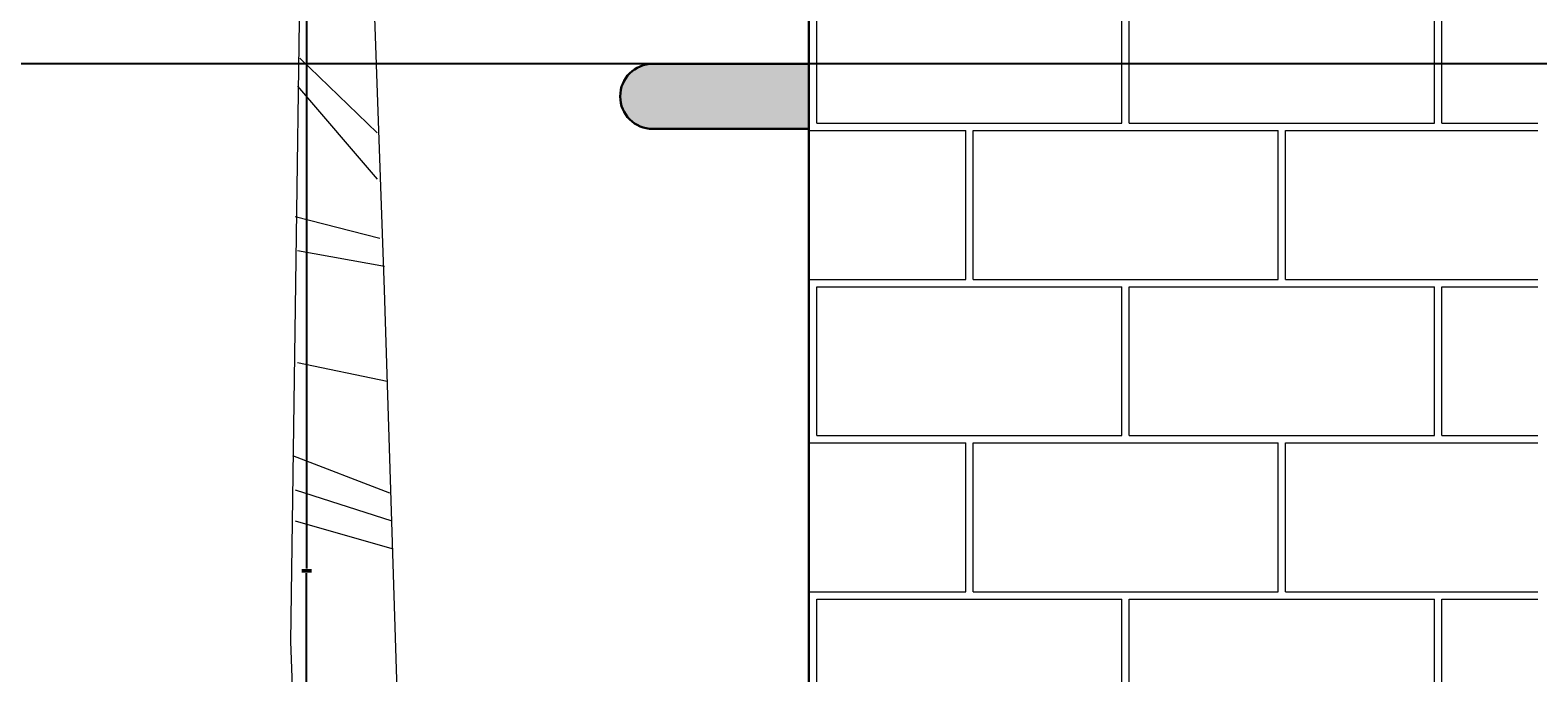
# Model space of a CAD drawing. Units: inches. Extents: x -301 to 715, y -607 to 364.
# Tile 129 of 141: x 194 to 310, y -440 to -391. Entities that reach past the tile are written whole.
import ezdxf

# ---------------------------------------------------------------- set-up
doc = ezdxf.new("R2010")
doc.units = ezdxf.units.IN
doc.header["$MEASUREMENT"] = 0
for name, color, linetype, lineweight in [('A-ANNO-DIMS', 2, 'Continuous', 18), ('A-ELEV', 220, 'Continuous', 30), ('A-ELEV-PATT', 4, 'Continuous', 13), ('L-PLNT', 94, 'Continuous', 13)]:
    doc.layers.add(name, color=color, linetype=linetype, lineweight=lineweight)
doc.styles.get("Standard").update_dxf_attribs({"font": 'arial.ttf'})
doc.dimstyles.get("Standard").update_dxf_attribs({"dimtxt": 0.18, "dimasz": 0.18, "dimexe": 0.18, "dimexo": 0.0625, "dimgap": 0.09, "dimtad": 0, "dimtih": 1, "dimtoh": 1, "dimdec": 1, "dimzin": 0, "dimdsep": 46, "dimlunit": 4, "dimtxsty": 'Standard', "dimcen": 0.09, "dimclrd": 3, "dimclre": 4, "dimclrt": 6, "dimadec": 0, "dimazin": 0, "dimtfac": 1, "dimtdec": 1, "dimtofl": 0, "dimtmove": 0, "dimatfit": 3, "dimfxl": 1, "dimtfill": 2, "dimtfillclr": 51, "dimtolj": 1, "dimtzin": 0, "dimarcsym": 0})

# ---------------------------------------------------------------- blocks, each defined once
blk = doc.blocks.new('*U34')
for p, q in [((-4.267, 114.428), (1.682, 108.708)), ((-4.453, 112.283), (1.682, 105.133)), ((-4.639, 102.273), (1.868, 100.604)), ((-4.453, 99.651), (2.24, 98.459)), ((-4.453, 91.071), (2.426, 89.641)), ((-4.825, 83.921), (2.612, 81.061)), ((-4.639, 81.299), (2.797, 78.916)), ((-4.639, 78.916), (2.797, 76.771))]:
    blk.add_line(p, q)
for points in [[(-2.363, 170.553), (-3.88, 148.505), (-4.988, 69.634), (-3.325, 24.869), (0, 0)], [(-0.116, 162.848), (0.554, 143.532), (2.217, 96.635), (3.88, 44.054), (7.76, 12.079), (11.64, 0)]]:
    blk.add_lwpolyline(points)
blk = doc.blocks.new('*D176')
at = {"layer": 'A-ANNO-DIMS', "color": 4, "lineweight": -2, "transparency": 16777216}
for p, q in [((148.28, -324.48), (215.61, -324.48)), ((-15.22, -540.48), (215.61, -540.48))]:
    blk.add_line(p, q, dxfattribs=at)
at = {"layer": 'A-ANNO-DIMS', "color": 3, "lineweight": -2, "transparency": 16777216}
for p, q in [((215.43, -324.66), (215.43, -432.3)), ((215.43, -540.3), (215.43, -432.66))]:
    blk.add_line(p, q, dxfattribs=at)
at = {"layer": 'A-ANNO-DIMS', "color": 3, "transparency": 16777216}
for points in [[(215.4, -324.66), (215.46, -324.66), (215.43, -324.48)], [(215.4, -540.3), (215.46, -540.3), (215.43, -540.48)]]:
    blk.add_solid(points, dxfattribs=at)
at = {"layer": 'Defpoints', "color": 0, "transparency": 16777216}
for p in [(148.22, -324.48), (-15.28, -540.48), (215.43, -540.48)]:
    blk.add_point(p, dxfattribs=at)
at = {"layer": 'A-ANNO-DIMS', "color": 6, "transparency": 16777216, "insert": (215.43, -432.48), "char_height": 0.18, "attachment_point": 5, "bg_fill": 1, "box_fill_scale": 1.25, "bg_fill_color": 51, "bg_fill_transparency": 0}
blk.add_mtext('\\A1;18\'-0"', dxfattribs=at)
blk = doc.blocks.new('*D200')
at = {"layer": 'A-ANNO-DIMS', "color": 4, "lineweight": -2, "transparency": 16777216}
for p, q in [((412.96, -393.55), (121.93, -393.55)), ((412.96, -489.55), (121.93, -489.55))]:
    blk.add_line(p, q, dxfattribs=at)
at = {"layer": 'A-ANNO-DIMS', "color": 3, "lineweight": -2, "transparency": 16777216}
for p, q in [((122.11, -393.73), (122.11, -441.37)), ((122.11, -489.37), (122.11, -441.73))]:
    blk.add_line(p, q, dxfattribs=at)
at = {"layer": 'A-ANNO-DIMS', "color": 3, "transparency": 16777216}
for points in [[(122.08, -393.73), (122.14, -393.73), (122.11, -393.55)], [(122.08, -489.37), (122.14, -489.37), (122.11, -489.55)]]:
    blk.add_solid(points, dxfattribs=at)
at = {"layer": 'Defpoints', "color": 0, "transparency": 16777216}
for p in [(122.11, -393.55), (413.02, -393.55), (413.02, -489.55)]:
    blk.add_point(p, dxfattribs=at)
at = {"layer": 'A-ANNO-DIMS', "color": 6, "transparency": 16777216, "insert": (122.11, -441.55), "char_height": 0.18, "attachment_point": 5, "bg_fill": 1, "box_fill_scale": 1.25, "bg_fill_color": 51, "bg_fill_transparency": 0}
blk.add_mtext('\\A1;8\'-0"', dxfattribs=at)

msp = doc.modelspace()

# ---------------------------------------------------------------- hatches: boundary and pattern name
at = {"layer": 'A-ELEV-PATT'}
h = msp.add_hatch(dxfattribs=at)
h.set_pattern_fill('AR-B816C', color=256, scale=1.5)
h.set_pattern_definition([(0, (458.621, 9.325), (12, 12), [23.4375, -0.5625]), (0, (446.621, 9.887), (12, 12), [23.4375, -0.5625]), (90, (458.621, 9.325), (-12, 12), [-12.5625, 11.4375]), (90, (458.059, 9.325), (-12, 12), [-12.5625, 11.4375])])
h.paths.add_polyline_path([(254.02, -489.55), (413.02, -489.55), (413.02, -393.55), (461.02, -393.55), (461.02, -489.55), (591.52, -489.55), (591.52, -369.55), (254.02, -369.55)])
h.paths.add_polyline_path([(310.02, -393.55), (360.02, -393.55), (360.02, -441.55), (310.02, -441.55)], flags=16)
h.paths.add_polyline_path([(315.02, -398.55), (355.02, -398.55), (355.02, -436.55), (315.02, -436.55)], flags=0)
h.paths.add_polyline_path([(496.77, -393.55), (546.77, -393.55), (546.77, -441.55), (496.77, -441.55)], flags=16)
h.paths.add_polyline_path([(501.77, -398.55), (541.77, -398.55), (541.77, -436.55), (501.77, -436.55)], flags=0)
h = msp.add_hatch(color=256, dxfattribs=at)
h.dxf.hatch_style = 1
h.paths.add_polyline_path([(242.02, -393.55, 1), (242.02, -398.55), (254.02, -398.55), (254.02, -393.55)])
h.paths.add_polyline_path([(603.52, -398.55, 1), (603.52, -393.55), (591.52, -393.55), (591.52, -398.55)])

# ---------------------------------------------------------------- linework, layer by layer
at = {"layer": 'A-ELEV'}
for p, q in [((254.02, -393.55), (242.02, -393.55)), ((254.02, -398.55), (242.02, -398.55))]:
    msp.add_line(p, q, dxfattribs=at)
msp.add_lwpolyline([(254.02, -369.55), (591.52, -369.55), (591.52, -489.55), (254.02, -489.55)], close=True, dxfattribs=at)
msp.add_arc((242.02, -396.05), 2.5, 90, 270, dxfattribs=at)

# ---------------------------------------------------------------- block references
at = {"layer": 'L-PLNT'}
msp.add_blockref('*U34', (219.18, -507.55), dxfattribs=at)

# ---------------------------------------------------------------- dimensions: what is measured, and where the dimension line sits
at = {"layer": 'A-ANNO-DIMS'}
for base, p1, p2, picture, middle in [((215.43, -540.48), (148.22, -324.48), (-15.28, -540.48), '*D176', (215.43, -432.48)), ((122.11, -393.55), (413.02, -489.55), (413.02, -393.55), '*D200', (122.11, -441.55))]:
    dim = msp.add_linear_dim(base=base, p1=p1, p2=p2, angle=90, dimstyle='Standard', override={"dimdec": 1, "dimlfac": 1, "dimrnd": 0, "dimzin": 1, "dimdsep": 46, "dimlunit": 4, "dimfrac": 2}, dxfattribs=at)
    dim.commit()
    dim.dimension.update_dxf_attribs({"geometry": picture, "text_midpoint": middle})

doc.saveas('drawing.dxf')
